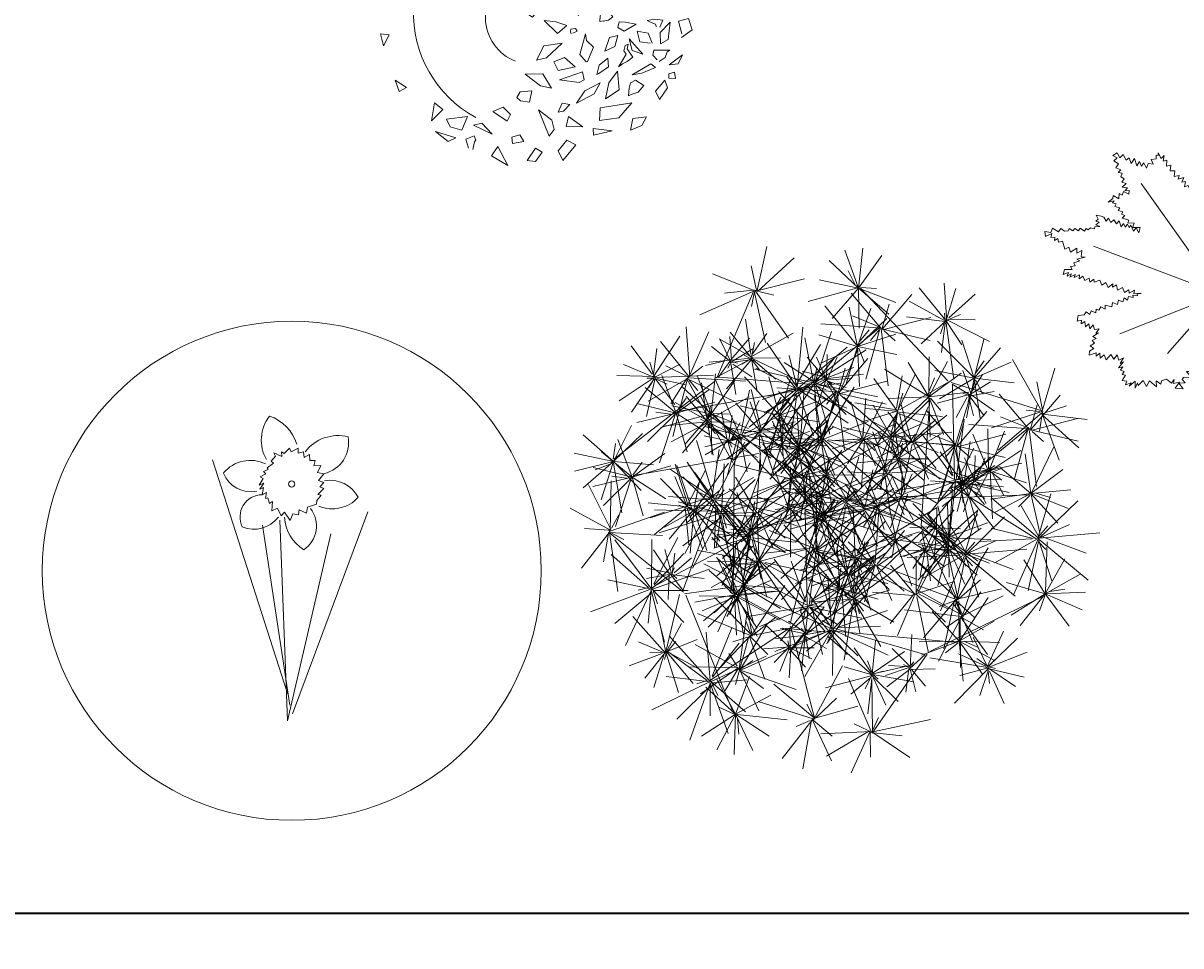
# Model space of a CAD drawing. Units: inches. Extents: x 8049 to 8459, y 820 to 1350.
# Tile 4 of 25: x 8102 to 8132, y 853 to 877. Entities that reach past the tile are written whole.
import ezdxf

# ---------------------------------------------------------------- set-up
doc = ezdxf.new("R2010")
doc.units = ezdxf.units.IN
doc.header["$MEASUREMENT"] = 0
for name, color, linetype, lineweight in [('A-ANNO-DIMS', 2, 'Continuous', 18), ('C-SITE-WALL', 7, 'Continuous', 35), ('zelen', 69, 'Continuous', 13)]:
    doc.layers.add(name, color=color, linetype=linetype, lineweight=lineweight)
doc.styles.get("Standard").update_dxf_attribs({"font": 'arial.ttf'})
doc.dimstyles.get("Standard").update_dxf_attribs({"dimtxt": 0.18, "dimasz": 0.18, "dimexe": 0.18, "dimexo": 0.0625, "dimgap": 0.09, "dimtad": 0, "dimtih": 1, "dimtoh": 1, "dimdec": 4, "dimzin": 0, "dimdsep": 46, "dimtxsty": 'Standard', "dimcen": 0.09, "dimadec": 0, "dimazin": 0, "dimtfac": 1, "dimtdec": 4, "dimtofl": 0, "dimtmove": 0, "dimatfit": 3, "dimfxl": 1, "dimtolj": 1, "dimtzin": 0, "dimarcsym": 0})

# ---------------------------------------------------------------- blocks, each defined once
blk = doc.blocks.new('z_08')
for p, q in [((-8.4, -246.7), (-159.3, 223.2)), ((1.5, -287.6), (152.7, 118.6)), ((-24, 101.7), (-8.7, -301.4)), ((-4.2, -270.1), (-58.8, 92)), ((-8.7, -301.4), (78.6, 74.5))]:
    blk.add_line(p, q)
blk.add_lwpolyline([(-36.3, 236.9), (-32.6, 230.3), (-41.2, 220.4), (-36.5, 216.2), (-49.7, 207), (-47.3, 203.9), (-56.6, 199.7), (-52.3, 194.9), (-63.8, 188.8), (-57.4, 185.2), (-65.8, 172.2), (-56.3, 176), (-64.1, 164.1), (-57, 167.5), (-59.7, 153), (-57.8, 153.7), (-50.7, 157.1), (-52.8, 145.2), (-48.1, 146.5), (-45, 135.3), (-38.5, 139.3), (-40.2, 120.4), (-28.8, 125.8), (-21.2, 110.3), (-14.4, 117.9), (-3.3, 101.4), (2, 114.8), (13.5, 112.2), (15.1, 122.7), (29.6, 116.1), (31.8, 127.6), (49.7, 133.8), (50.1, 141.4), (58.8, 151.7), (52.1, 153.6), (64.2, 165.2), (56.2, 168.6), (64.4, 177.6), (53.7, 181.6), (64.6, 194.7), (51.7, 197.5), (58.1, 211.7), (44.3, 211.1), (47, 222), (36.1, 222), (35.4, 233.6), (25.1, 227.9), (23.8, 239.3), (13.1, 236.2), (12.5, 246.7), (-1.1, 239.3), (-4.7, 246.4), (-15.5, 235.7), (-20.6, 239.4), (-19.7, 229.8), (-36.3, 236.9)])
for centre, radius in [((0, 0), 501.6), ((-0.3, 174.4), 6.32)]:
    blk.add_circle(centre, radius)
for centre, radius, start, end in [((18.1, 262.8), 79.4, 142.6945, 209.6234), ((-71.1, 230.6), 84.5, 16.4392, 72.0686), ((92.3, 189.3), 82.4, 75.3361, 142.797), ((51, 257.3), 63.3, 282.6991, 10.6878), ((-83.4, 151.9), 70, 63.8597, 140.3167), ((-82.2, 217.5), 58.9, 200.8344, 281.4173), ((76.9, 117.5), 64.4, 27.9746, 99.6629), ((-59.4, 108.2), 44.7, 90.8466, 206.078), ((81.2, 195.8), 71.2, 247.7997, 317.4677), ((-7.1, 90), 56.9, 303.1089, 38.3983), ((-75.6, 144.7), 61, 246.9504, 322.7891), ((70, 113.9), 85.1, 184.0633, 237.2607)]:
    blk.add_arc(centre, radius, start, end)
blk = doc.blocks.new('z_85')
for p, q in [((168.5, 483.9), (169.7, 507.5)), ((169.7, 507.5), (194.7, 497.5)), ((140.4, 459.9), (144.1, 478.3)), ((144.1, 478.3), (154.8, 474.2)), ((154.8, 474.2), (155.6, 493.8)), ((155.6, 493.8), (168.5, 483.9)), ((194.7, 497.5), (173, 491.4)), ((173, 491.4), (185.2, 481.2)), ((185.2, 481.2), (186.9, 458.5)), ((-334.5, 433), (-320.5, 441.8)), ((-320.5, 441.8), (-312.2, 426.3)), ((-312.2, 426.3), (-302, 436.4)), ((-302, 436.4), (-292.5, 418.9)), ((-192.6, 433.8), (-192.5, 442.2)), ((-192.5, 442.2), (-183.3, 424.5)), ((-2.1, 435.8), (11.7, 434.9)), ((11.4, 414.5), (-2.1, 435.8)), ((8.4, 449), (15.4, 438)), ((11.7, 434.9), (8.4, 449)), ((15.4, 438), (25.6, 455.6)), ((25.6, 455.6), (26.4, 439.7)), ((26.4, 439.7), (44.1, 447.4)), ((44.1, 447.4), (54.4, 436.3)), ((54.4, 436.3), (52.3, 421.7)), ((98.5, 438.8), (116.6, 438)), ((108.9, 418.4), (98.5, 438.8)), ((116.1, 450.2), (130, 447.6)), ((116.6, 438), (116.1, 450.2)), ((130, 447.6), (130.9, 460.7)), ((130.9, 460.7), (140.4, 459.9)), ((185.1, 447.3), (169, 438)), ((169, 438), (186.4, 430.3)), ((186.9, 458.5), (172.1, 453.2)), ((172.1, 453.2), (185.1, 447.3)), ((-320.3, 426.3), (-334.5, 433)), ((-331, 417), (-320.3, 426.3)), ((-316.9, 407.2), (-331, 417)), ((-325.3, 394.5), (-316.9, 407.2)), ((-292.5, 418.9), (-282.7, 426.1)), ((-282.7, 426.1), (-277, 408.1)), ((-277, 408.1), (-266.3, 423.5)), ((-266.3, 423.5), (-258.7, 400.7)), ((-258.7, 400.7), (-250.8, 414.2)), ((-250.8, 414.2), (-244.9, 399.8)), ((-244.9, 399.8), (-237.2, 410.8)), ((-237.2, 410.8), (-228.5, 393.9)), ((-228.5, 393.9), (-223.5, 408.6)), ((-223.5, 408.6), (-207.8, 406.4)), ((-214.2, 421.3), (-198.5, 423)), ((-207.8, 406.4), (-214.2, 421.3)), ((-198.5, 423), (-198.2, 434.1)), ((-198.2, 434.1), (-192.6, 433.8)), ((-183.3, 424.5), (-173.3, 433.2)), ((-173.3, 433.2), (-176.4, 415.5)), ((-176.4, 415.5), (-165.1, 418.9)), ((-165.1, 418.9), (-166.4, 400.3)), ((-166.4, 400.3), (-152.4, 402.8)), ((-152.4, 402.8), (-154.8, 385.2)), ((-10.8, 396), (-9.6, 410.9)), ((-9.6, 410.9), (-3.8, 416.9)), ((-3.8, 416.9), (11.4, 414.5)), ((52.3, 421.7), (64.6, 426)), ((64.6, 426), (59.8, 403.9)), ((59.8, 403.9), (75.6, 414.2)), ((75.6, 414.2), (88.3, 401.4)), ((86.4, 422.5), (108.9, 418.4)), ((88.3, 401.4), (86.4, 422.5)), ((186.4, 430.3), (169.1, 422.7)), ((169.1, 422.7), (188.1, 417.5)), ((183.6, 400.7), (169.1, 387.1)), ((188.1, 417.5), (174.5, 406.5)), ((174.5, 406.5), (183.6, 400.7)), ((-309.5, 388.7), (-325.3, 394.5)), ((-317.2, 380.4), (-309.5, 388.7)), ((-305.1, 378.2), (-317.2, 380.4)), ((-309.5, 366.8), (-305.1, 378.2)), ((-299.2, 360.3), (-309.5, 366.8)), ((-154.8, 385.2), (-139.8, 385.6)), ((-139.8, 385.6), (-142, 367.5)), ((-142, 367.5), (-126.8, 370.7)), ((-126.8, 370.7), (-129.7, 358.9)), ((-129.7, 358.9), (-112.6, 364.1)), ((-112.6, 364.1), (-118.7, 349.7)), ((-31.2, 364.3), (-16.4, 364.7)), ((-19.6, 354.2), (-31.2, 364.3)), ((-19.9, 378.2), (-4.1, 379.1)), ((-16.4, 364.7), (-19.9, 378.2)), ((-4.1, 379.1), (-10.8, 396)), ((0, 0), (132.7, 397)), ((182.7, 383.5), (168.5, 371)), ((168.5, 371), (185.5, 367.5)), ((169.1, 387.1), (182.7, 383.5)), ((185.5, 367.5), (169.7, 351.3)), ((169.7, 351.3), (191.1, 364.1)), ((191.1, 364.1), (194, 345.3)), ((-305.9, 349.8), (-299.2, 360.3)), ((-292.6, 345.9), (-305.9, 349.8)), ((-305.3, 333.9), (-292.6, 345.9)), ((-288.9, 332.3), (-305.3, 333.9)), ((-296.8, 323.1), (-288.9, 332.3)), ((0, 0), (-245.8, 345.3)), ((-118.7, 349.7), (-106.5, 351.7)), ((-106.5, 351.7), (-110.4, 335.8)), ((-110.4, 335.8), (-98.6, 339.2)), ((-98.6, 339.2), (-92.9, 326.8)), ((-92.9, 326.8), (-89.6, 322.3)), ((-61.6, 314), (-48.8, 329.6)), ((-48.8, 329.6), (-45, 336.2)), ((-45, 336.2), (-26.1, 337)), ((-37.5, 352.7), (-19.6, 354.2)), ((-26.1, 337), (-37.5, 352.7)), ((194, 345.3), (206.3, 360.8)), ((206.3, 360.8), (201.7, 341.2)), ((201.7, 341.2), (224.8, 344.2)), ((224.8, 344.2), (203.2, 339.2)), ((203.2, 339.2), (217.5, 321.8)), ((-348.8, 287.5), (-334.3, 298.5)), ((-329.7, 291.9), (-348.8, 287.5)), ((-335.7, 285.2), (-329.7, 291.9)), ((-334.3, 298.5), (-333.4, 308.7)), ((-333.4, 308.7), (-315.2, 298.3)), ((-315.2, 298.3), (-314.9, 314.1)), ((-314.9, 314.1), (-305, 309.4)), ((-305, 309.4), (-300.9, 321)), ((-300.9, 321), (-284.3, 312.7)), ((-283.1, 324), (-296.8, 323.1)), ((-284.3, 312.7), (-283.1, 324)), ((-89.6, 322.3), (-91.1, 309)), ((-91.1, 309), (-80.4, 316.3)), ((-80.4, 316.3), (-81.2, 298.5)), ((-81.2, 298.5), (-70.2, 306.6)), ((-70.2, 306.6), (-73.6, 287.8)), ((-73.6, 287.8), (-62, 294.6)), ((-62, 294.6), (-51.7, 290.2)), ((-51.7, 290.2), (-61.6, 314)), ((199.8, 290.5), (179.5, 286.4)), ((204.7, 306.3), (183.1, 303.2)), ((183.1, 303.2), (199.8, 290.5)), ((217.5, 321.8), (196.8, 317.3)), ((196.8, 317.3), (204.7, 306.3)), ((-323.9, 282.5), (-335.7, 285.2)), ((-327.7, 273.4), (-323.9, 282.5)), ((-312.5, 269.8), (-327.7, 273.4)), ((-318.1, 260.9), (-312.5, 269.8)), ((-303.5, 257.1), (-318.1, 260.9)), ((-306.9, 250.2), (-303.5, 257.1)), ((187.9, 258.2), (158.6, 247.3)), ((198, 276.2), (169.3, 269.4)), ((169.3, 269.4), (187.9, 258.2)), ((179.5, 286.4), (198, 276.2)), ((305.4, 235.8), (330.6, 255.3)), ((330.6, 255.3), (314, 234.4)), ((-387.5, 216.4), (-377.3, 224.9)), ((-387.2, 228.2), (-380.3, 234.1)), ((-377.3, 224.9), (-387.2, 228.2)), ((-386.6, 246.8), (-370.9, 243.8)), ((-380.3, 234.1), (-386.6, 246.8)), ((-370.9, 243.8), (-362.5, 240.1)), ((-362.5, 240.1), (-355.4, 227.7)), ((-355.4, 227.7), (-347.7, 237.1)), ((-347.7, 237.1), (-340.1, 223.9)), ((-340.1, 223.9), (-331.2, 232.1)), ((-331.2, 232.1), (-323, 219.9)), ((-323, 219.9), (-314.9, 229.4)), ((-314.9, 229.4), (-308.7, 210.5)), ((-308.7, 210.5), (-301.4, 220.5)), ((-296.5, 245.4), (-306.9, 250.2)), ((-304.8, 236.9), (-296.5, 245.4)), ((-284, 230.8), (-304.8, 236.9)), ((-301.4, 220.5), (-296.2, 209.5)), ((-296.2, 209.5), (-288.7, 218.5)), ((-288.7, 218.5), (-282.8, 208)), ((-287.5, 222.7), (-284, 230.8)), ((-267.9, 221.3), (-287.5, 222.7)), ((-272.7, 208.1), (-267.9, 221.3)), ((166.6, 220), (142.5, 215.8)), ((169.1, 234), (156.5, 228.6)), ((156.5, 228.6), (166.6, 220)), ((158.6, 247.3), (176.5, 239.3)), ((176.5, 239.3), (169.1, 234)), ((225, 203.7), (227.4, 221.4)), ((227.4, 221.4), (237.6, 211.9)), ((237.6, 211.9), (244, 229.6)), ((244, 229.6), (251.2, 218.3)), ((251.2, 218.3), (269.1, 241.8)), ((269.1, 241.8), (276.1, 228.2)), ((276.1, 228.2), (284.6, 245.4)), ((291.9, 231.3), (282.8, 224.3)), ((282.8, 224.3), (297.7, 215.3)), ((284.6, 245.4), (292.5, 230.8)), ((294, 233.8), (291.9, 231.3)), ((292.5, 230.8), (304.2, 252.6)), ((314, 234.4), (294, 233.8)), ((304.2, 252.6), (305.4, 235.8)), ((-547.4, 195.4), (-527.9, 192.6)), ((-544.7, 179.5), (-547.4, 195.4)), ((-524.7, 189.5), (-544.7, 179.5)), ((-528.5, 176.6), (-524.7, 189.5)), ((-527.9, 192.6), (-523, 206.4)), ((-523, 206.4), (-504.7, 194.2)), ((-504.7, 194.2), (-496.5, 204.8)), ((-496.5, 204.8), (-486, 196.2)), ((-486, 196.2), (-473.8, 197.3)), ((-473.8, 197.3), (-470.6, 205)), ((-470.6, 205), (-459, 197.9)), ((-459, 197.9), (-453.2, 204.7)), ((-453.2, 204.7), (-441.7, 197.3)), ((-441.7, 197.3), (-436, 206.1)), ((-436, 206.1), (-423, 196.7)), ((-423, 196.7), (-417.9, 205.5)), ((-417.9, 205.5), (-411.3, 200.8)), ((-411.3, 200.8), (-403.9, 207.3)), ((-403.9, 207.3), (-392, 203.9)), ((-392, 203.9), (-391, 210.5)), ((-391, 210.5), (-375.1, 210.9)), ((-375.1, 210.9), (-387.5, 216.4)), ((-282.8, 208), (-278.3, 215.3)), ((-278.3, 215.3), (-269.6, 197)), ((-249.1, 208.6), (-272.7, 208.1)), ((-269.6, 197), (-261.6, 206.7)), ((-261.6, 206.7), (-252.6, 191.1)), ((-252.6, 191.1), (-249.1, 208.6)), ((157.5, 207.7), (133, 198.3)), ((133, 198.3), (152.7, 194.8)), ((152.7, 194.8), (134.2, 181.8)), ((134.2, 181.8), (152.3, 190.3)), ((142.5, 215.8), (157.5, 207.7)), ((152.3, 190.3), (165.5, 178.4)), ((165.5, 178.4), (166.1, 202.2)), ((166.1, 202.2), (195.8, 210)), ((195.8, 210), (206.3, 202.3)), ((206.3, 202.3), (214.9, 212.7)), ((214.9, 212.7), (225, 203.7)), ((297.7, 215.3), (285.2, 201.4)), ((285.2, 201.4), (305.7, 207.8)), ((305.7, 207.8), (318.4, 196.7)), ((318.4, 196.7), (331.5, 207.2)), ((331.5, 207.2), (343.4, 195.3)), ((343.4, 195.3), (349.2, 197.8)), ((349.2, 197.8), (357.1, 191.7)), ((357.1, 191.7), (363.4, 194)), ((363.4, 194), (375.4, 187.3)), ((375.4, 187.3), (381.6, 192.9)), ((381.6, 192.9), (391.6, 185.1)), ((391.6, 185.1), (399.5, 189.8)), ((399.5, 189.8), (410.7, 177.1)), ((410.7, 177.1), (423.8, 189)), ((423.8, 189), (430.9, 177.3)), ((430.9, 177.3), (445.2, 185.4)), ((445.2, 185.4), (440.2, 166.6)), ((-515.5, 177.6), (-528.5, 176.6)), ((-516.7, 167.9), (-515.5, 177.6)), ((-506.3, 173.2), (-516.7, 167.9)), ((-504.7, 162.4), (-506.3, 173.2)), ((-491.4, 165.7), (-504.7, 162.4)), ((-484.9, 140.6), (-491.4, 165.7)), ((-472, 147), (-484.9, 140.6)), ((-466.4, 131.1), (-472, 147)), ((0, 0), (-394.4, 149.4)), ((422.9, 156), (399.8, 152.7)), ((399.8, 152.7), (410.7, 140.5)), ((410.7, 167.7), (422.9, 156)), ((431.6, 161.5), (410.7, 167.7)), ((423.8, 175.6), (431.6, 161.5)), ((440.2, 166.6), (423.8, 175.6)), ((-447.4, 143.9), (-466.4, 131.1)), ((-446.4, 127.5), (-447.4, 143.9)), ((-447.3, 109), (-420.9, 115.7)), ((-437.9, 103.7), (-447.3, 109)), ((-431.2, 136.1), (-446.4, 127.5)), ((-433.6, 116.8), (-432.5, 124.7)), ((-420.9, 115.7), (-433.6, 116.8)), ((-432.5, 124.7), (-431.2, 136.1)), ((0, 0), (313.9, 140.8)), ((392.9, 111.3), (367, 110.4)), ((367, 110.4), (384, 100.5)), ((370, 124.5), (392.9, 111.3)), ((397.4, 117.9), (370, 124.5)), ((380.7, 131.9), (397.4, 117.9)), ((402.3, 129), (380.7, 131.9)), ((410.7, 140.5), (391.1, 138)), ((391.1, 138), (402.3, 129)), ((-490.1, 61.5), (-485.7, 76.6)), ((-485.7, 76.6), (-461.1, 77.2)), ((-466.3, 86.6), (-452.6, 88.2)), ((-461.1, 77.2), (-466.3, 86.6)), ((-456.8, 97.3), (-437.9, 103.7)), ((-452.6, 88.2), (-456.8, 97.3)), ((367.5, 85.5), (348.2, 79.7)), ((348.2, 79.7), (364, 72.5)), ((367.3, 93.6), (352.7, 93.5)), ((352.7, 93.5), (367.5, 85.5)), ((354.4, 102.3), (367.3, 93.6)), ((384, 100.5), (354.4, 102.3)), ((364, 72.5), (355.3, 62.8)), ((-472.7, 67.7), (-490.1, 61.5)), ((-477.3, 56.2), (-472.7, 67.7)), ((-464.1, 63.3), (-477.3, 56.2)), ((-468.4, 52.6), (-464.1, 63.3)), ((-452, 61.1), (-468.4, 52.6)), ((-455.1, 51.2), (-452, 61.1)), ((-439, 59.8), (-455.1, 51.2)), ((-439.5, 47.5), (-439, 59.8)), ((-428.5, 56.1), (-439.5, 47.5)), ((-421.5, 42.4), (-428.5, 56.1)), ((-408.4, 49.5), (-421.5, 42.4)), ((-406.6, 37.3), (-408.4, 49.5)), ((-393.5, 46.8), (-406.6, 37.3)), ((-392.2, 37), (-393.5, 46.8)), ((-375.3, 43.4), (-392.2, 37)), ((-368.7, 27.4), (-375.3, 43.4)), ((-356.3, 36.3), (-368.7, 27.4)), ((-348.5, 20.8), (-356.3, 36.3)), ((355.3, 62.8), (346.4, 53.6)), ((346.4, 53.6), (362.3, 46.4)), ((362.3, 46.4), (350.4, 40.1)), ((350.4, 40.1), (365.4, 35.2)), ((-333.9, 32.3), (-348.5, 20.8)), ((-335.5, 21.5), (-333.9, 32.3)), ((-322.4, 29.1), (-335.5, 21.5)), ((-319.9, 12.2), (-322.4, 29.1)), ((-303.8, 20), (-319.9, 12.2)), ((0, 0), (-312.2, -125)), ((-297.7, 5.3), (-303.8, 20)), ((-284.2, 12.8), (-297.7, 5.3)), ((-282.8, 2.5), (-284.2, 12.8)), ((-266.1, 11.6), (-282.8, 2.5)), ((-268.5, 0.9), (-266.1, 11.6)), ((-245.2, 1.9), (-268.5, 0.9)), ((-258.6, 1.3), (-245.2, 1.9)), ((-256.6, -5.5), (-258.6, 1.3)), ((0, 0), (-163.1, -186)), ((0, 0), (249.7, -43.2)), ((365.4, 35.2), (364.6, 26)), ((364.6, 26), (373.9, 25.2)), ((373.9, 25.2), (368.8, 14.6)), ((368.8, 14.6), (381.5, 13.5)), ((381.5, 13.5), (372.3, 1.1)), ((372.3, 1.1), (390.8, -3.1)), ((-358.6, -35.2), (-337, -39.8)), ((-358.3, -47.6), (-358.6, -35.2)), ((-337, -39.8), (-335.4, -26.5)), ((-335.4, -26.5), (-320, -32.7)), ((-320, -32.7), (-316.6, -19.6)), ((-316.6, -19.6), (-303.5, -24.4)), ((-303.5, -24.4), (-299.1, -12.1)), ((-299.1, -12.1), (-288.4, -18.9)), ((-288.4, -18.9), (-284.9, -7.8)), ((-284.9, -7.8), (-270.6, -10.5)), ((-272, -3.8), (-256.6, -5.5)), ((-270.6, -10.5), (-272, -3.8)), ((14.2, -31.5), (3.8, -40.4)), ((11, -15.5), (4.4, -23.3)), ((4.4, -23.3), (14.2, -31.5)), ((19.4, -9.1), (6, -11.1)), ((20.6, -19.7), (19.4, -9.1)), ((34.5, -21), (20.6, -19.7)), ((33.9, -27.7), (34.5, -21)), ((44.7, -33.5), (33.9, -27.7)), ((43.2, -50.4), (44.7, -33.5)), ((352.1, -22.6), (362.5, -39.2)), ((365.2, -32.7), (352.1, -22.6)), ((368.7, -23.2), (365.2, -32.7)), ((380.7, -30.1), (368.7, -23.2)), ((390.8, -3.1), (374.2, -7.2)), ((374.2, -7.2), (396.2, -16.9)), ((378.3, -17.7), (377.9, -21.9)), ((377.9, -21.9), (380.7, -30.1)), ((396.2, -16.9), (378.3, -17.7)), ((-445.6, -85.2), (-442.8, -66.9)), ((-442.8, -66.9), (-423.6, -64.7)), ((-423.6, -64.7), (-418.1, -55.3)), ((-418.1, -55.3), (-406.6, -63.9)), ((-406.6, -63.9), (-402.1, -52.8)), ((-402.1, -52.8), (-387.5, -58.3)), ((-387.5, -58.3), (-386, -47.3)), ((-386, -47.3), (-378.3, -50.6)), ((-378.3, -50.6), (-371.8, -40.4)), ((-371.8, -40.4), (-358.3, -47.6)), ((3.8, -40.4), (23.3, -42)), ((23.3, -42), (17.8, -55.3)), ((17.8, -55.3), (33.3, -57.2)), ((35.8, -67.3), (26.2, -78.5)), ((33.3, -57.2), (27.6, -66.1)), ((27.6, -66.1), (35.8, -67.3)), ((57.8, -49.8), (43.2, -50.4)), ((57.8, -66.7), (57.8, -49.8)), ((79.4, -63.3), (57.8, -66.7)), ((80.6, -68.6), (79.4, -63.3)), ((95, -77.7), (80.6, -68.6)), ((362.5, -39.2), (352.9, -44.5)), ((352.9, -44.5), (372.4, -54.8)), ((372.4, -54.8), (362.2, -67.3)), ((362.2, -67.3), (377.4, -74.9)), ((-431.8, -81.7), (-445.6, -85.2)), ((-433, -93.3), (-431.8, -81.7)), ((-421.5, -86.1), (-433, -93.3)), ((-420.3, -102.3), (-421.5, -86.1)), ((-408.9, -93.6), (-420.3, -102.3)), ((-406.5, -108.7), (-408.9, -93.6)), ((-396.2, -96.8), (-406.5, -108.7)), ((-391.4, -111), (-396.2, -96.8)), ((-377.3, -108.5), (-391.4, -111)), ((-387.6, -122.5), (-377.3, -108.5)), ((35.4, -79.2), (20.9, -86.9)), ((20.9, -86.9), (36.1, -88.5)), ((26.2, -78.5), (35.4, -79.2)), ((36.1, -88.5), (28.2, -99.3)), ((28.2, -99.3), (46.8, -102.9)), ((46.8, -102.9), (31.9, -112.9)), ((96.5, -95.7), (95, -77.7)), ((114.9, -96.9), (96.5, -95.7)), ((113.9, -113.2), (114.9, -96.9)), ((259.9, -104.5), (278.9, -118.5)), ((281.6, -108.4), (259.9, -104.5)), ((279.1, -92.7), (281.6, -108.4)), ((288.4, -105.6), (279.1, -92.7)), ((292.3, -97.7), (288.4, -105.6)), ((306.3, -109.8), (292.3, -97.7)), ((312.3, -101.9), (306.3, -109.8)), ((319.1, -112.6), (312.3, -101.9)), ((329.4, -104.1), (319.1, -112.6)), ((341.7, -115.9), (329.4, -104.1)), ((350.6, -106.3), (341.7, -115.9)), ((357.5, -125.6), (350.6, -106.3)), ((377.4, -74.9), (371.4, -84.3)), ((371.4, -84.3), (390.2, -87.1)), ((390.2, -87.1), (391, -98.7)), ((391, -98.7), (403.6, -97.7)), ((403.6, -97.7), (399.4, -115.7)), ((-399.4, -144.9), (-386, -138.6)), ((-391.7, -153.5), (-399.4, -144.9)), ((-396.7, -133.3), (-378.8, -121.8)), ((-386, -138.6), (-396.7, -133.3)), ((-378.8, -121.8), (-387.6, -122.5)), ((31.9, -112.9), (31.3, -114)), ((31.3, -114), (51.4, -114.8)), ((49.4, -132), (38, -139.7)), ((38, -139.7), (55.7, -140.9)), ((51.4, -114.8), (39.8, -130.3)), ((39.8, -130.3), (49.4, -132)), ((55.7, -140.9), (40.8, -150.5)), ((131.6, -109.3), (113.9, -113.2)), ((129.5, -124.2), (131.6, -109.3)), ((150, -116), (129.5, -124.2)), ((153.5, -138.6), (150, -116)), ((168.2, -134.7), (153.5, -138.6)), ((168.7, -151.1), (168.2, -134.7)), ((278.9, -118.5), (264.8, -122.8)), ((264.8, -122.8), (279.4, -131.9)), ((280.4, -134.4), (275.3, -145.6)), ((279.4, -131.9), (280.4, -134.4)), ((375.9, -109.5), (357.5, -125.6)), ((386.6, -123.9), (375.9, -109.5)), ((403.8, -118.5), (386.6, -123.9)), ((399.4, -115.7), (414.2, -115.6)), ((413.1, -135.8), (403.8, -118.5)), ((414.2, -115.6), (406.2, -120.7)), ((406.2, -120.7), (430, -130.9)), ((430, -130.9), (413.1, -135.8)), ((-408.7, -191.2), (-407.1, -178.7)), ((-407.1, -178.7), (-394, -170.7)), ((-405.7, -161.9), (-391.7, -153.5)), ((-394, -170.7), (-405.7, -161.9)), ((57.1, -178.7), (40.5, -191.1)), ((40.8, -150.5), (61.7, -147.7)), ((57.7, -166.9), (43.5, -179.6)), ((43.5, -179.6), (57.1, -178.7)), ((67.9, -157.4), (45.5, -166.6)), ((45.5, -166.6), (57.7, -166.9)), ((61.7, -147.7), (51.2, -158.2)), ((51.2, -158.2), (67.9, -157.4)), ((187.2, -147), (168.7, -151.1)), ((190.4, -171.9), (187.2, -147)), ((199.5, -167.6), (190.4, -171.9)), ((201.2, -183.5), (199.5, -167.6)), ((215.4, -180.2), (201.2, -183.5)), ((214.3, -200.6), (215.4, -180.2)), ((273.9, -166.2), (257.2, -175.1)), ((257.2, -175.1), (270.6, -182.1)), ((279.5, -153.9), (259.5, -159.1)), ((259.5, -159.1), (273.9, -166.2)), ((275.3, -145.6), (279.5, -153.9)), ((-386.3, -183.7), (-408.7, -191.2)), ((-386.9, -194.2), (-386.3, -183.7)), ((-375, -185.4), (-386.9, -194.2)), ((-374.4, -200.4), (-375, -185.4)), ((-361, -190), (-374.4, -200.4)), ((-355.6, -205.5), (-361, -190)), ((-340.1, -188.9), (-355.6, -205.5)), ((-331, -204.2), (-340.1, -188.9)), ((-320.5, -190.1), (-331, -204.2)), ((-315.8, -206.4), (-320.5, -190.1)), ((-316.4, -230.7), (-301.2, -212.5)), ((-300.9, -199.4), (-315.8, -206.4)), ((-311, -217.5), (-300.9, -199.4)), ((-301.2, -212.5), (-311, -217.5)), ((-78.5, -215.2), (-63.4, -228.2)), ((-63.1, -216.4), (-78.5, -215.2)), ((-64.5, -193.4), (-63.1, -216.4)), ((-54.1, -209.7), (-64.5, -193.4)), ((-39.9, -196.5), (-54.1, -209.7)), ((-40.4, -212.5), (-39.9, -196.5)), ((-25.3, -207.7), (-40.4, -212.5)), ((-25.3, -223.8), (-25.3, -207.7)), ((-10.7, -215.8), (-25.3, -223.8)), ((-8.3, -228.6), (-10.7, -215.8)), ((40.5, -191.1), (53.9, -190.4)), ((53.9, -190.4), (47.9, -199)), ((47.9, -199), (63.4, -198.7)), ((65.1, -205.6), (53.6, -216.1)), ((53.6, -216.1), (64.9, -216.9)), ((64.9, -216.9), (56, -222.4)), ((63.4, -198.7), (65.1, -205.6)), ((229.7, -192.5), (214.3, -200.6)), ((235.5, -207.5), (229.7, -192.5)), ((253.5, -202), (235.5, -207.5)), ((255.4, -217.1), (253.5, -202)), ((270.6, -214.1), (255.4, -217.1)), ((270.6, -182.1), (255.6, -190.7)), ((255.6, -190.7), (268.7, -194.5)), ((268.7, -194.5), (256, -201.4)), ((256, -201.4), (270.6, -214.1)), ((-303, -227.7), (-316.4, -230.7)), ((-309.9, -238.3), (-303, -227.7)), ((-298.3, -242.6), (-309.9, -238.3)), ((-304.7, -251.3), (-298.3, -242.6)), ((-295, -254.3), (-304.7, -251.3)), ((-79.8, -242), (-103.3, -242.6)), ((-103.3, -242.6), (-88.9, -260)), ((-63.4, -228.2), (-87.9, -229.1)), ((-87.9, -229.1), (-79.8, -242)), ((8.9, -223.5), (-8.3, -228.6)), ((12.7, -238.7), (8.9, -223.5)), ((24.7, -230.5), (12.7, -238.7)), ((23, -244.8), (24.7, -230.5)), ((35.5, -238.8), (23, -244.8)), ((40.7, -254.5), (35.5, -238.8)), ((49.8, -244.9), (40.7, -254.5)), ((52.7, -259.2), (49.8, -244.9)), ((63.6, -245.9), (52.7, -259.2)), ((56, -222.4), (69.4, -226.9)), ((69.4, -226.9), (58.1, -234.3)), ((58.1, -234.3), (70.9, -234.4)), ((72.4, -265), (63.6, -245.9)), ((73.9, -233.5), (67.9, -243.4)), ((67.9, -243.4), (79.4, -252.4)), ((79.4, -252.4), (68.2, -253.9)), ((70.9, -234.4), (73.9, -233.5)), ((-305.3, -270.9), (-295, -254.3)), ((-290.1, -273.1), (-305.3, -270.9)), ((-294.6, -284.2), (-290.1, -273.1)), ((-277.1, -277.7), (-294.6, -284.2)), ((-264.9, -273), (-283.1, -288.1)), ((-283.1, -288.1), (-277.1, -277.7)), ((-264.3, -294.3), (-264.9, -273)), ((-256.6, -277.5), (-264.3, -294.3)), ((-254.5, -286.6), (-256.6, -277.5)), ((-239.6, -270.1), (-254.5, -286.6)), ((-228.6, -289.1), (-239.6, -270.1)), ((-220, -272), (-228.6, -289.1)), ((-197.9, -289.9), (-220, -272)), ((-199.2, -272), (-197.9, -289.9)), ((-184.2, -282), (-199.2, -272)), ((-182.4, -271.4), (-184.2, -282)), ((-166.3, -266.5), (-182.4, -271.4)), ((-151.2, -278.6), (-166.3, -266.5)), ((-142.3, -267.5), (-151.2, -278.6)), ((-144.6, -280.3), (-142.3, -267.5)), ((-126.2, -276.2), (-144.6, -280.3)), ((-138.9, -294.9), (-126.2, -276.2)), ((-107.8, -278), (-127.3, -279.2)), ((-127.3, -279.2), (-114.3, -296.8)), ((-113.1, -261.1), (-117.3, -267.5)), ((-117.3, -267.5), (-107.8, -278)), ((-88.9, -260), (-113.1, -261.1)), ((68.2, -253.9), (72.4, -265)), ((-114.3, -296.8), (-138.9, -294.9))]:
    blk.add_line(p, q)
blk = doc.blocks.new('z_66')
for p, q in [((83.2, 488.9), (72.7, 477.7)), ((72.7, 477.7), (96.4, 469.7)), ((129.8, 476.2), (83.2, 488.9)), ((134, 464.6), (129.8, 476.2)), ((-176.4, 458.5), (-191.7, 438.6)), ((-191.7, 438.6), (-165.6, 433.5)), ((-139.2, 449.4), (-176.4, 458.5)), ((-165.6, 433.5), (-163.6, 441.1)), ((-161.1, 434.6), (-139.2, 449.4)), ((-13.6, 463.6), (-42.5, 459.2)), ((-42.5, 459.2), (-39.3, 446.9)), ((-30.3, 449.4), (-13.6, 463.6)), ((96.4, 469.7), (114.5, 463.9)), ((114.5, 463.9), (114.5, 463.9)), ((120.4, 457.8), (134, 464.6)), ((-254, 399.9), (-283.6, 397.7)), ((-272.8, 380.7), (-254, 399.9)), ((-165.6, 433.5), (-165.6, 433.5)), ((-138.9, 404.9), (-156.9, 400.2)), ((-156.9, 400.2), (-153.8, 385.4)), ((-133.3, 394.8), (-138.9, 404.9)), ((265.2, 432.1), (258.2, 407.5)), ((258.2, 407.5), (287.4, 387.2)), ((258.2, 407.5), (281.9, 388.6)), ((287.4, 387.2), (265.2, 432.1)), ((-283.6, 397.7), (-297.2, 378.2)), ((-297.2, 378.2), (-277.7, 376)), ((-277.7, 376), (-272.8, 380.7)), ((-241.9, 321.7), (-199.1, 397.3)), ((-231.4, 383.6), (-241.9, 321.7)), ((-199.1, 397.3), (-231.4, 383.6)), ((-148.6, 384.7), (-133.3, 394.8)), ((281.9, 388.6), (281.9, 388.6)), ((-330.3, 328.9), (-298.6, 327.1)), ((-316, 288.8), (-330.3, 328.9)), ((-298.6, 327.1), (-280.8, 297.1)), ((344.2, 293.1), (292, 357.2)), ((292, 357.2), (326.8, 341.2)), ((326.8, 341.2), (344.2, 293.1)), ((-280.8, 297.1), (-316, 288.8)), ((383.1, 281.9), (364.4, 316.3)), ((364.4, 316.3), (394.6, 305.1)), ((394.6, 305.1), (383.1, 281.9)), ((-377.9, 259.1), (-399.2, 252.6)), ((-358.4, 254), (-377.9, 259.1)), ((-356, 217.5), (-358.4, 254)), ((350.8, 280.8), (348.7, 270.3)), ((348.7, 270.3), (358.8, 264.5)), ((369.2, 266.7), (350.8, 280.8)), ((358.8, 264.5), (358.8, 264.5)), ((363.3, 256.6), (369.2, 266.7)), ((-399.2, 252.6), (-405.8, 224)), ((-405.8, 224), (-368.2, 216.4)), ((400.9, 251.9), (393.9, 214.6)), ((426.6, 192.2), (400.9, 251.9)), ((-396.4, 196.1), (-438.1, 150.2)), ((-414.8, 150.9), (-396.4, 196.1)), ((-368.2, 216.4), (-368.2, 216.4)), ((348, 215.7), (356, 188.9)), ((395.3, 193.2), (348, 215.7)), ((356, 188.9), (395.3, 193.2)), ((393.9, 214.6), (426.6, 192.2)), ((-438.1, 150.2), (-414.8, 150.9)), ((225.2, 159.9), (197, 140.8)), ((256.8, 142.6), (225.2, 159.9)), ((323.6, 157.8), (297.5, 149.8)), ((297.5, 149.8), (314.6, 119.4)), ((314.6, 119.4), (352.9, 145.5)), ((352.9, 145.5), (323.6, 157.8)), ((450, 180.6), (434.3, 171.2)), ((434.3, 171.2), (449.6, 142.6)), ((449.6, 142.6), (467.7, 160.3)), ((467.7, 160.3), (450, 180.6)), ((197, 140.8), (249.5, 113.6)), ((249.5, 113.6), (256.8, 142.6)), ((336.9, 84.3), (405.8, 131.7)), ((405.8, 131.7), (389.8, 82.1)), ((-468.4, 91.6), (-466.3, 62.6)), ((-441.6, 89), (-468.4, 91.6)), ((-458.3, 53.9), (-421.1, 76)), ((-421.1, 76), (-441.6, 89)), ((164.3, 94.8), (154.2, -2.2)), ((178.9, 33.3), (164.3, 94.8)), ((193.1, 101.3), (238, 52.1)), ((261.7, 66.6), (193.1, 101.3)), ((265.2, 98.8), (297.2, 42.7)), ((318.8, 66.2), (265.2, 98.8)), ((372.7, 93), (336.9, 84.3)), ((389.8, 82.1), (372.7, 93)), ((441.6, 95.9), (420.7, 86.5)), ((420.7, 86.5), (440.2, 78.5)), ((440.2, 78.5), (459.7, 59.7)), ((470.5, 93.7), (441.6, 95.9)), ((463.2, 57.9), (474, 73.5)), ((474, 73.5), (470.5, 93.7)), ((-466.3, 62.6), (-466.3, 62.6)), ((238, 52.1), (261.7, 66.6)), ((297.2, 42.7), (294.1, 53.6)), ((297.2, 42.7), (318.8, 66.2)), ((347.3, 45.2), (332.7, 18.1)), ((376.9, 52.5), (347.3, 45.2)), ((350.8, 10.9), (376.9, 52.5)), ((459.7, 59.7), (459.7, 59.7)), ((11.8, 6.2), (0, 0)), ((0, 0), (12.2, -6.9)), ((12.2, -6.9), (19.1, 2.9)), ((19.1, 2.9), (15.7, 5.8)), ((154.2, -2.2), (178.9, 33.3)), ((229, 7.2), (223.1, -2.5)), ((250.6, 9.8), (229, 7.2)), ((263.4, -5.4), (250.6, 9.8)), ((332.7, 18.1), (350.8, 10.9)), ((84.6, -21.7), (48, -17)), ((48, -17), (90.1, -58.3)), ((119.4, -32.9), (84.6, -21.7)), ((90.1, -58.3), (119.4, -32.9)), ((223.1, -2.5), (222.7, -20.6)), ((222.7, -20.6), (234.2, -18.1)), ((233.2, -19.9), (249.9, -15.9)), ((234.2, -18.1), (234.2, -18.1)), ((249.9, -15.9), (263.4, -5.4)), ((282.9, -21.3), (279.1, -39.1)), ((302.1, -22.8), (282.9, -21.3)), ((298.6, -50.3), (335.8, -28.6)), ((335.8, -28.6), (302.1, -22.8)), ((393.6, -13), (371, -17)), ((371, -17), (383.5, -23.5)), ((383.5, -23.5), (396.7, -28.9)), ((420, -15.9), (393.6, -13)), ((396.7, -28.9), (398.5, -35.5)), ((398.5, -35.5), (399.5, -35.8)), ((410.3, -38), (420, -15.9)), ((442, -22.4), (411.3, -55.4)), ((436, -77.1), (442, -22.4)), ((499.7, -10.9), (468.8, -19.9)), ((468.8, -19.9), (478.8, -58.6)), ((510.9, -47), (499.7, -10.9)), ((-464.2, -59.3), (-436.4, -62.6)), ((-454.5, -96.3), (-464.2, -59.3)), ((-436.4, -62.6), (-454.5, -96.3)), ((131.9, -44.9), (130.2, -52.5)), ((130.2, -52.5), (132.9, -59.3)), ((146.5, -42.3), (131.9, -44.9)), ((138.2, -56.8), (151, -51)), ((151, -51), (146.5, -42.3)), ((177.8, -59), (160.1, -123.8)), ((181, -80.3), (177.8, -59)), ((252.6, -70.9), (237.7, -112.9)), ((278.4, -64), (252.6, -70.9)), ((269.7, -98.4), (278.4, -64)), ((279.1, -39.1), (298.6, -50.3)), ((339, -51), (347.7, -84.3)), ((374.1, -56.8), (339, -51)), ((386.3, -87.9), (374.1, -56.8)), ((411.3, -55.4), (412.7, -90.8)), ((477.5, -70.2), (510.9, -47)), ((478.8, -58.6), (478.8, -58.6)), ((47.7, -96.6), (24, -141.9)), ((104.1, -87.9), (47.7, -96.6)), ((56, -133.9), (104.1, -87.9)), ((202.2, -100.6), (181, -80.3)), ((183.7, -145.5), (202.2, -100.6)), ((237.7, -112.9), (269.7, -98.4)), ((301.7, -95.5), (297.9, -112.2)), ((310.8, -91.9), (301.7, -95.5)), ((307.6, -106), (310.8, -91.9)), ((325.4, -132.4), (307.6, -106)), ((314.2, -74.2), (356.7, -123)), ((323.3, -111.1), (314.2, -74.2)), ((347.7, -84.3), (379.7, -88.3)), ((379.7, -88.3), (379.7, -88.3)), ((391.2, -110), (393.2, -108.6)), ((412.7, -90.8), (436, -77.1)), ((24, -141.9), (56, -133.9)), ((111.4, -132.8), (78.3, -146.2)), ((145.1, -162.1), (111.4, -132.8)), ((160.1, -123.8), (179.6, -146.6)), ((247.1, -135.7), (220.6, -157)), ((249.2, -162.1), (247.1, -135.7)), ((304.5, -123), (291.6, -145.8)), ((297.9, -112.2), (304.5, -123)), ((308.3, -145.8), (325.4, -132.4)), ((356.7, -123), (323.3, -111.1)), ((356.7, -123), (356.7, -123)), ((356.7, -123), (356.7, -123)), ((391.2, -110), (388.4, -125.6)), ((388.4, -125.6), (402.3, -140.8)), ((441.3, -110), (391.2, -110)), ((402.3, -140.8), (402.3, -140.8)), ((407.9, -145.5), (427, -133.5)), ((427, -133.5), (432.9, -115.8)), ((432.9, -115.8), (441.3, -110)), ((480.9, -124.5), (439.2, -156)), ((467.7, -153.4), (480.9, -124.5)), ((78.3, -146.2), (92.2, -174.1)), ((92.2, -174.1), (145.1, -162.1)), ((168.1, -178.4), (96.7, -202.6)), ((173, -203.4), (168.1, -178.4)), ((179.6, -146.6), (183.7, -145.5)), ((220.6, -157), (212.6, -186)), ((219.2, -183.5), (249.2, -162.1)), ((277.4, -176.2), (250.2, -212.4)), ((283.3, -233.8), (277.4, -176.2)), ((291.6, -145.8), (281.2, -161.8)), ((281.2, -161.8), (293, -152.7)), ((293, -152.7), (308.3, -145.8)), ((382.5, -152.7), (323.3, -187.4)), ((353.9, -182), (396.7, -164.3)), ((396.7, -164.3), (382.5, -152.7)), ((438.5, -183.8), (456.2, -179.1)), ((439.2, -156), (467.7, -153.4)), ((456.2, -179.1), (458.7, -199)), ((-417.9, -204.1), (-405.1, -239.6)), ((-382.8, -226.5), (-417.9, -204.1)), ((44.5, -184.2), (-10.8, -184.9)), ((-10.8, -184.9), (36.9, -222.2)), ((71, -229.1), (44.5, -184.2)), ((96.7, -202.6), (157.6, -211.3)), ((157.6, -211.3), (173, -203.4)), ((223.8, -212.4), (175.4, -237.7)), ((204.3, -246.8), (223.8, -212.4)), ((212.6, -186), (219.2, -183.5)), ((250.2, -212.4), (240.1, -262.4)), ((318.4, -212.1), (314.6, -228.7)), ((334.1, -203.7), (318.4, -212.1)), ((323.3, -187.4), (353.9, -182)), ((360.2, -221.1), (334.1, -203.7)), ((425.3, -204.5), (396.7, -238.5)), ((434.3, -228), (425.3, -204.5)), ((438.5, -197.6), (438.5, -183.8)), ((458.7, -199), (438.5, -197.6)), ((-405.1, -239.6), (-382.8, -226.5)), ((-26.4, -240.3), (-37.6, -258.4)), ((10.1, -237.7), (-26.4, -240.3)), ((2.4, -273.2), (10.1, -237.7)), ((36.9, -222.2), (71, -229.1)), ((175.4, -237.7), (149.6, -276.1)), ((149.6, -276.1), (204.3, -246.8)), ((240.1, -262.4), (283.3, -233.8)), ((314.6, -228.7), (311.8, -252.6)), ((311.8, -252.6), (320.5, -249.3)), ((320.5, -249.3), (342.8, -241.4)), ((342.8, -241.4), (360.2, -221.1)), ((396.7, -238.5), (409.2, -264.2)), ((409.2, -264.2), (434.3, -228)), ((-295.1, -275), (-304.2, -331.5)), ((-269, -296), (-295.1, -275)), ((-80, -288), (-112.4, -302.5)), ((-56.7, -311.6), (-80, -288)), ((-37.6, -258.4), (-25.8, -268.5)), ((-25.8, -268.5), (2.4, -273.2)), ((-25.8, -268.5), (-25.8, -268.5)), ((-25.8, -268.5), (-25.8, -268.5)), ((105.1, -276.1), (91.9, -303.6)), ((128.8, -280.4), (105.1, -276.1)), ((108.6, -301.4), (128.8, -280.4)), ((322.2, -275), (223.8, -290.2)), ((282.2, -321.7), (322.2, -275)), ((-304.2, -331.5), (-269, -296)), ((-191.1, -317.4), (-256.8, -326.4)), ((-209.8, -360.4), (-191.1, -317.4)), ((-112.4, -302.5), (-67.5, -331.8)), ((-67.5, -331.8), (-56.7, -311.6)), ((30.6, -297.1), (72.7, -329.3)), ((64, -379.6), (30.6, -297.1)), ((91.9, -303.6), (108.6, -301.4)), ((117.3, -348.8), (124.2, -317.7)), ((124.2, -317.7), (168.8, -349.9)), ((223.8, -290.2), (221.3, -330)), ((221.3, -330), (282.2, -321.7)), ((325.7, -323.9), (318.4, -360.1)), ((368.9, -319.2), (325.7, -323.9)), ((354.3, -346.3), (368.9, -319.2)), ((-256.8, -326.4), (-245.7, -350.3)), ((-245.7, -350.3), (-209.8, -360.4)), ((-172.6, -344.9), (-146.9, -338.7)), ((-114.8, -372.7), (-172.6, -344.9)), ((-146.9, -338.7), (-114.8, -372.7)), ((79.3, -357.9), (64, -379.6)), ((72.7, -329.3), (79.3, -357.9)), ((168.8, -349.9), (117.3, -348.8)), ((201.8, -355), (202.2, -376.3)), ((261, -362.2), (201.8, -355)), ((318.4, -360.1), (354.3, -346.3)), ((-292, -364.4), (-252, -395.5)), ((-228.3, -383.9), (-292, -364.4)), ((-252, -395.5), (-228.3, -383.9)), ((-197.3, -388.3), (-171.2, -377.8)), ((-188.3, -416.9), (-197.3, -388.3)), ((-169.5, -396.6), (-174.7, -420.5)), ((-171.2, -377.8), (-166, -391.5)), ((-166, -391.5), (-169.5, -396.6)), ((-27.8, -374.5), (-52.9, -381.8)), ((-52.9, -381.8), (-50.8, -402)), ((-50.8, -402), (-15.3, -396.2)), ((-15.3, -396.2), (-27.8, -374.5)), ((91.9, -424.8), (119, -391.5)), ((119, -391.5), (146.9, -406.4)), ((202.2, -376.3), (261, -362.2)), ((-174.7, -420.5), (-174.7, -420.5)), ((-116.2, -441.1), (-96.4, -411.8)), ((-96.4, -411.8), (-65.8, -470.8)), ((21.6, -417.2), (-4.5, -455.6)), ((42.1, -428.8), (21.6, -417.2)), ((21.6, -458.1), (42.1, -428.8)), ((106.8, -455.6), (91.9, -424.8)), ((146.9, -406.4), (106.8, -455.6)), ((-65.8, -470.8), (-116.2, -441.1)), ((-4.5, -455.6), (21.6, -458.1))]:
    blk.add_line(p, q)
for centre, radius, start, end in [((11.8, 6.2), 372.3, 50.2118, 241.5185), ((12.2, -6.9), 147.8, 46.7611, 248.9067)]:
    blk.add_arc(centre, radius, start, end)
blk = doc.blocks.new('z_96')
for p, q in [((-279.8, 149.9), (-254.2, 304.5)), ((-277.5, 143.8), (-209, 319.2)), ((-2.3, 183.5), (-55.4, 292.1)), ((0.6, 181.7), (29.5, 299.6)), ((-282.5, 143.4), (-440.4, 263.7)), ((-279.3, 139.9), (-326.8, 270.9)), ((1.7, 182.4), (-92.5, 262.1)), ((3.6, 188.7), (58.7, 265.3)), ((5.7, 184.9), (91.8, 284.8)), ((-276.5, 141.1), (-146.8, 221.3)), ((-9.6, 182.8), (-129.6, 222.9)), ((395.6, 94.6), (438.6, 246.5)), ((-5.7, 186.4), (-99.8, 114.3)), ((-4.6, 181.6), (-86.6, 72.3)), ((-0.6, 184.6), (125.7, 194.4)), ((1.5, 182.8), (69.9, 77.5)), ((9.8, 182.3), (88, 114.6)), ((393.4, 89.6), (354, 209.2)), ((393.4, 89.6), (479.1, 181.8)), ((-292.1, 134.2), (-430.8, 180.4)), ((-280.1, 150.3), (-304, 174)), ((-260.4, 142.3), (-97.9, 156.1)), ((-4.6, -3.2), (0.8, 176.4)), ((393.4, 89.6), (284.7, 153.1)), ((-283.2, 138.5), (-471.2, 114.9)), ((-279.1, 142.3), (-397.9, 16.9)), ((-285.6, 136.6), (-375, 92.2)), ((-277.6, 139.7), (-313.4, -1.1)), ((-279.1, 135.4), (-307.4, 99.5)), ((-278.4, 130.6), (-221.9, 40)), ((-277.5, 137.2), (-129.1, 19.3)), ((-17.8, -5.6), (-274.7, 141.8)), ((-263.2, 140.3), (-131, 113.5)), ((393.4, 89.6), (514.5, 123.6)), ((0, 0), (389.1, 84.4)), ((393.4, 89.6), (273.9, 50.1)), ((393.4, 89.6), (293.9, 12.5)), ((391.3, 83.5), (363.2, 41.9)), ((393.4, 89.6), (493.5, 13.4)), ((393.4, 89.6), (516.7, 64.5)), ((393.4, 89.6), (442.6, -26.2)), ((409.2, 93.4), (456.4, 89)), ((-74.7, -24.6), (-111.9, 37.5)), ((-71.7, -35.5), (-42.1, 65.4)), ((164.1, -89.9), (142.7, 11.7)), ((163.4, -89), (238.9, 7.6)), ((-237.5, -199.4), (-267, -22)), ((-10.4, -6), (-235.7, -205.3)), ((-74, -33), (-152.4, -40.5)), ((-65.2, -32.9), (-135.5, -11.4)), ((-76.2, -35.8), (-103.5, -105.8)), ((-80, -28.7), (-89.9, -20)), ((-16, -6.1), (-74.7, -37.4)), ((-72.5, -35.1), (-71.9, -112)), ((-68.1, -28.4), (-55.8, -19.3)), ((-5, -18.9), (163.8, -91.6)), ((159.3, -86.3), (85.5, -28.7)), ((167, -88.4), (276, -24.7)), ((-234, -202.3), (-196.3, -40.6)), ((-75, -39.2), (-157.1, -75.4)), ((-70.4, -41.1), (3.7, -57.1)), ((-69.9, -39.6), (-38.4, -102.6)), ((163.4, -86.5), (137.7, -55.7)), ((168.3, -88.4), (194, -71.5)), ((167.1, -94.6), (37.3, -175)), ((161.1, -92.4), (74, -95.2)), ((163.6, -101.8), (119, -170.9)), ((164.5, -93.4), (157.3, -141.4)), ((160.4, -93), (267.6, -148.2)), ((164.2, -92.2), (234.3, -170.2)), ((165.3, -92), (295.7, -74)), ((166.9, -90.5), (187.1, -100.1)), ((167, -104.1), (188, -212.9)), ((-237.4, -199.3), (-392.1, -169)), ((-246.4, -194), (-283.1, -163.8)), ((-231, -196), (-205.2, -161.9)), ((-242.3, -196.3), (-391.5, -241.3)), ((-242.2, -199.4), (-329.5, -310.3)), ((-241, -201.7), (-259.1, -277.3)), ((-242.2, -201.7), (-47.9, -207.3)), ((-236.2, -200.9), (-139.2, -306.8)), ((-230.8, -205.8), (-146.5, -236))]:
    blk.add_line(p, q)
blk = doc.blocks.new('сосна 1')
for p, rotation in [((317.7, 388.3), 121.1570021628385), ((-412.6, 386.5), 205.4822314301707), ((-117.1, 122.3), 55.05972244949475), ((-136.5, 361.1), 177.7388340989747), ((-351.5, 121.7), 257.3134436407499), ((285.8, 9.1), 60.73020616460848), ((-143.1, -5.5), 121.1570021628385), ((234.4, -65.1), 73.8676290404427), ((-343.1, -101.5), 57.88453704712605), ((-274, 161.3), 177.7388340989747), ((173.8, 17), 349.7944254651076), ((326.9, 45.9), 177.7388340989747), ((98.1, -4.6), 177.7388340989747), ((-502.4, -282.3), 279.7984529833926), ((-175.3, -367), 63.19571700542104), ((-48.9, -393.6), 342.5348703671633), ((260.9, -458.6), 13.72293452966709)]:
    blk.add_blockref('z_96', p, dxfattribs=dict(rotation=rotation))
blk = doc.blocks.new('*D70')
at = {"layer": 'A-ANNO-DIMS', "color": 0, "lineweight": -2, "transparency": 16777216}
for p, q in [((8083.397, 1045.808), (8083.397, 820.091)), ((8137.397, 1045.808), (8137.397, 820.091)), ((8083.577, 820.271), (8110.179, 820.271)), ((8137.217, 820.271), (8110.616, 820.271))]:
    blk.add_line(p, q, dxfattribs=at)
at = {"layer": 'A-ANNO-DIMS', "color": 0, "transparency": 16777216}
for points in [[(8083.577, 820.301), (8083.577, 820.241), (8083.397, 820.271)], [(8137.217, 820.301), (8137.217, 820.241), (8137.397, 820.271)]]:
    blk.add_solid(points, dxfattribs=at)
at = {"layer": 'Defpoints', "color": 0, "transparency": 16777216}
for p in [(8083.397, 1045.871), (8137.397, 1045.871), (8083.397, 820.271)]:
    blk.add_point(p, dxfattribs=at)
at = {"layer": 'A-ANNO-DIMS', "color": 0, "transparency": 16777216, "insert": (8110.397, 820.271), "char_height": 0.18, "attachment_point": 5}
blk.add_mtext('\\A1;54', dxfattribs=at)
blk = doc.blocks.new('*D76')
at = {"layer": 'A-ANNO-DIMS', "color": 0, "lineweight": -2, "transparency": 16777216}
for p, q in [((8083.397, 1054.808), (8083.397, 820.091)), ((8299.397, 1054.808), (8299.397, 820.091)), ((8083.577, 820.271), (8191.107, 820.271)), ((8299.217, 820.271), (8191.688, 820.271))]:
    blk.add_line(p, q, dxfattribs=at)
at = {"layer": 'A-ANNO-DIMS', "color": 0, "transparency": 16777216}
for points in [[(8083.577, 820.301), (8083.577, 820.241), (8083.397, 820.271)], [(8299.217, 820.301), (8299.217, 820.241), (8299.397, 820.271)]]:
    blk.add_solid(points, dxfattribs=at)
at = {"layer": 'Defpoints', "color": 0, "transparency": 16777216}
for p in [(8083.397, 1054.871), (8299.397, 1054.871), (8299.397, 820.271)]:
    blk.add_point(p, dxfattribs=at)
at = {"layer": 'A-ANNO-DIMS', "color": 0, "transparency": 16777216, "insert": (8191.397, 820.271), "char_height": 0.18, "attachment_point": 5}
blk.add_mtext('\\A1;216', dxfattribs=at)
blk = doc.blocks.new('*D88')
at = {"layer": 'A-ANNO-DIMS', "color": 0, "lineweight": -2, "transparency": 16777216}
for p, q in [((8083.397, 1162.808), (8083.397, 820.091)), ((8139.397, 1162.808), (8139.397, 820.091)), ((8083.577, 820.271), (8111.179, 820.271)), ((8139.217, 820.271), (8111.616, 820.271))]:
    blk.add_line(p, q, dxfattribs=at)
at = {"layer": 'A-ANNO-DIMS', "color": 0, "transparency": 16777216}
for points in [[(8083.577, 820.301), (8083.577, 820.241), (8083.397, 820.271)], [(8139.217, 820.301), (8139.217, 820.241), (8139.397, 820.271)]]:
    blk.add_solid(points, dxfattribs=at)
at = {"layer": 'Defpoints', "color": 0, "transparency": 16777216}
for p in [(8083.397, 1162.871), (8139.397, 1162.871), (8139.397, 820.271)]:
    blk.add_point(p, dxfattribs=at)
at = {"layer": 'A-ANNO-DIMS', "color": 0, "transparency": 16777216, "insert": (8111.397, 820.271), "char_height": 0.18, "attachment_point": 5}
blk.add_mtext('\\A1;56', dxfattribs=at)

msp = doc.modelspace()

# ---------------------------------------------------------------- linework, layer by layer
at = {"layer": 'C-SITE-WALL'}
msp.add_line((8083.3974, 853.8706), (8219.8974, 853.8706), dxfattribs=at)

# ---------------------------------------------------------------- block references
at = {"layer": 'zelen'}
for name, p, xscale, yscale, zscale in [('z_66', (8115.2411, 877.0978), 0.0082668533249786, 0.0082668533249786, 0.0082668533249786), ('z_85', (8133.1125, 869.8806), 0.0082668533249786, 0.0082668533249786, 0.0082668533249786), ('сосна 1', (8123.4579, 864.4267), 0.0082668533249786, 0.0082668533249786, 0.0082668533249786), ('z_08', (8109.112, 862.7233), 0.0128650146468131, 0.0128650146468131, 0.0128650146468131)]:
    msp.add_blockref(name, p, dxfattribs=dict(at, xscale=xscale, yscale=yscale, zscale=zscale))

# ---------------------------------------------------------------- dimensions: what is measured, and where the dimension line sits
at = {"layer": 'A-ANNO-DIMS'}
for base, p1, p2, picture, middle in [((8139.3974, 820.2706), (8083.3974, 1162.8706), (8139.3974, 1162.8706), '*D88', (8111.3974, 820.2706)), ((8299.3974, 820.2706), (8083.3974, 1054.8706), (8299.3974, 1054.8706), '*D76', (8191.3974, 820.2706)), ((8083.3974, 820.2706), (8137.3974, 1045.8706), (8083.3974, 1045.8706), '*D70', (8110.3974, 820.2706))]:
    dim = msp.add_linear_dim(base=base, p1=p1, p2=p2, dimstyle='Standard', override={"dimdec": 0, "dimlfac": 1, "dimrnd": 0, "dimzin": 0, "dimdsep": 46, "dimlunit": 2}, dxfattribs=at)
    dim.commit()
    dim.dimension.update_dxf_attribs({"geometry": picture, "text_midpoint": middle})

doc.saveas('drawing.dxf')
